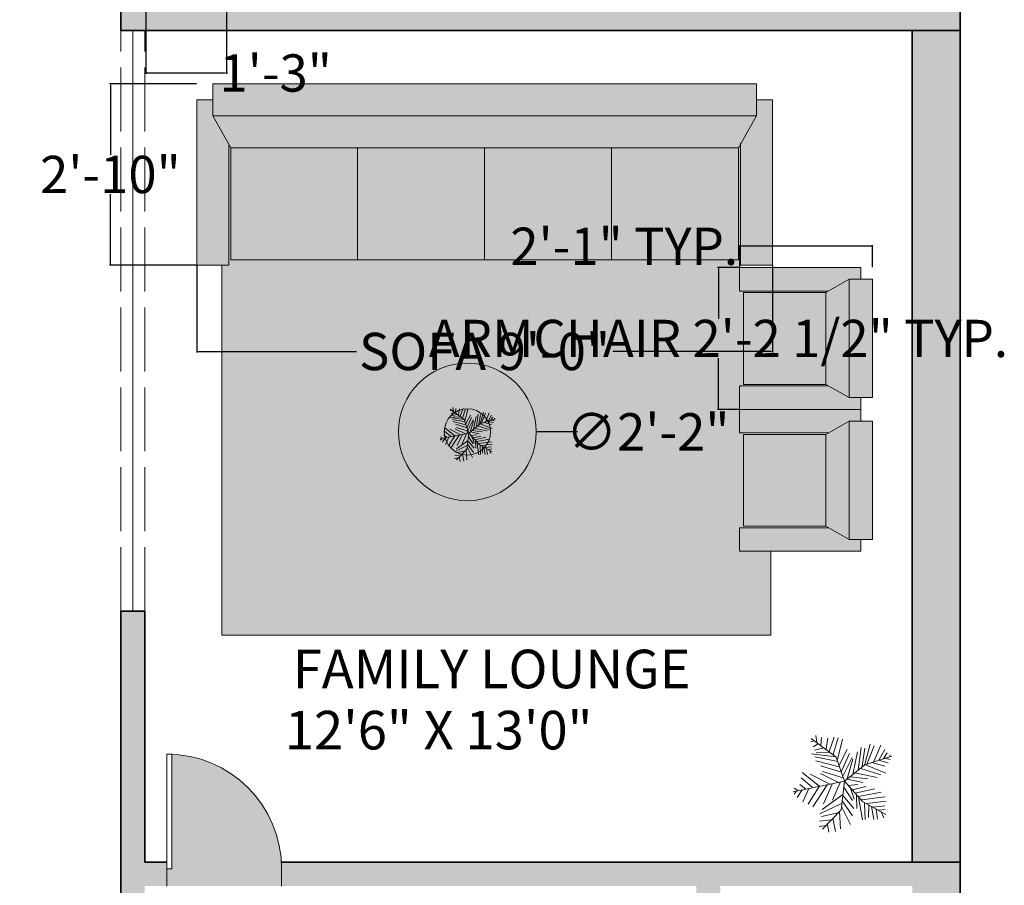
# Model space of a CAD drawing. Units: inches. Extents: x 2167 to 2589, y 1680 to 2489.
# Tile 33 of 38: x 2399 to 2583, y 1865 to 2027. Entities that reach past the tile are written whole.
import ezdxf

# ---------------------------------------------------------------- set-up
doc = ezdxf.new("R2010")
doc.units = ezdxf.units.IN
doc.header["$MEASUREMENT"] = 0
doc.linetypes.add('ACAD_ISO02W100', pattern=[15, 12, -3])
doc.layers.get('0').update_dxf_attribs({"color": 250})
for name, color, linetype, lineweight in [('A-ANNO-DIMS', 2, 'Continuous', 18), ('A-AREA-IDEN', 7, 'Continuous', 18), ('A-DOOR', 4, 'Continuous', 18), ('A-FURN-PATT', 31, 'Continuous', 13), ('A-WALL-OVHD', 8, 'ACAD_ISO02W100', 18), ('A-WALL-PATT', 250, 'Continuous', 13), ('C-PROP', 7, 'Continuous', 35), ('furniture', 34, 'Continuous', 18), ('L-PLNT', 106, 'Continuous', 13), ('walls', 7, 'Continuous', 35), ('windows', 141, 'Continuous', 18)]:
    doc.layers.add(name, color=color, linetype=linetype, lineweight=lineweight)
doc.layers.add('A-FLOR-PATT', color=254, linetype='Continuous', lineweight=13, true_color=0xfeeab9)
doc.styles.get("Standard").update_dxf_attribs({"font": 'arial.ttf'})
doc.dimstyles.get("Standard").update_dxf_attribs({"dimtxt": 7, "dimasz": 0.18, "dimexe": 0.18, "dimexo": 0.0625, "dimgap": 0.09, "dimtad": 0, "dimtih": 1, "dimtoh": 1, "dimdec": 1, "dimzin": 0, "dimdsep": 46, "dimlunit": 3, "dimtxsty": 'Standard', "dimcen": 0.09, "dimadec": 0, "dimazin": 0, "dimtfac": 1, "dimtdec": 1, "dimtofl": 0, "dimtmove": 0, "dimatfit": 3, "dimfxl": 1, "dimtolj": 1, "dimtzin": 0, "dimarcsym": 0})

# ---------------------------------------------------------------- blocks, each defined once
blk = doc.blocks.new('*U2')
for p, q in [((0, 0), (0, -6)), ((40, 0), (40, -6))]:
    blk.add_line(p, q)
blk.add_lwpolyline([(0, 0), (0, 40), (1.75, 40), (1.75, 0)], close=True)
blk.add_arc((0, 0), 40, 0, 90)
blk = doc.blocks.new('FABRIC SOFA 4S')
at = {"layer": 'furniture'}
for p, q in [((3, 54), (34, 54)), ((3, 51), (3, 54)), ((34, 48), (34, 54)), ((0, -51), (0, 51)), ((6, 51), (0, 51)), ((6, -51), (6, 51)), ((12, 47.63), (6, 51)), ((11.14, 48), (34, 48)), ((33, 23.81), (12, 23.81)), ((33, 0), (12, 0)), ((33, -23.81), (12, -23.81)), ((6, -51), (12, -47.63)), ((11.54, -48), (34, -48)), ((34, -48), (34, -54)), ((6, -51), (0, -51)), ((3, -54), (3, -51)), ((3, -54), (34, -54))]:
    blk.add_line(p, q, dxfattribs=at)
blk.add_lwpolyline([(12, -47.63), (12, 47.63), (33, 47.63), (33, -47.63)], close=True, dxfattribs=at)
blk = doc.blocks.new('FABRIC SOFA 1S')
at = {"layer": 'furniture'}
for p, q in [((3, 18.12), (34, 18.12)), ((3, 15.12), (3, 18.12)), ((34, 12.12), (34, 18.12)), ((0, -15.12), (0, 15.12)), ((6, 15.12), (0, 15.12)), ((6, -15.12), (6, 15.12)), ((12, 11.75), (6, 15.12)), ((11.33, 12.12), (34, 12.12)), ((6, -15.12), (12, -11.75)), ((11.33, -12.12), (34, -12.12)), ((34, -12.12), (34, -18.12)), ((6, -15.12), (0, -15.12)), ((3, -18.12), (3, -15.12)), ((3, -18.12), (34, -18.12))]:
    blk.add_line(p, q, dxfattribs=at)
blk.add_lwpolyline([(12, -11.75), (12, 11.75), (33, 11.75), (33, -11.75)], close=True, dxfattribs=at)
blk = doc.blocks.new('*U8')
for p, q in [((-10.186, 53.64), (-13.084, 55.962)), ((0, 0), (-10.5, 57)), ((-9.099, 51.782), (-6.563, 55.962)), ((-7.288, 39.707), (-21.778, 46.673)), ((-8.737, 47.138), (-17.069, 52.711)), ((-7.65, 43.423), (-2.578, 49.46)), ((-5.839, 35.992), (4.667, 48.067)), ((-5.114, 27.632), (10.463, 46.673)), ((-3.665, 19.273), (-27.574, 35.527)), ((-5.114, 28.097), (-24.676, 40.636)), ((-2.941, 16.486), (8.652, 37.85)), ((27, 9), (48, 36)), ((27.127, 9.056), (31.112, 35.992)), ((35.096, 32.741), (37.27, 22.524)), ((38.719, 34.134), (41.979, 28.561)), ((44.153, 36.456), (45.239, 32.741)), ((-31.5, 4.5), (-52.5, 25.5)), ((-48.585, 21.131), (-49.309, 29.026)), ((-43.513, 28.561), (-42.427, 15.558)), ((-38.442, 26.239), (-34.819, 7.663)), ((-35.544, 28.097), (-24.314, 3.947)), ((-14.533, 2.09), (-30.834, 25.31)), ((-24.314, 23.917), (-2.941, 13.7)), ((-1.129, 6.734), (9.014, 26.704)), ((3.942, 1.625), (11.187, 24.381)), ((10.101, 3.483), (17.708, 26.239)), ((16.259, 5.805), (23.142, 31.348)), ((22.055, 7.198), (27.489, 32.277)), ((31.836, 30.883), (32.561, 16.486)), ((40.53, 25.775), (48.862, 24.846)), ((43.791, 29.954), (51.036, 30.883)), ((-47.498, 19.737), (-55.83, 18.344)), ((-40.615, 13.7), (-55.105, 10.913)), ((-20.691, 13.7), (-1.129, 4.876)), ((29.662, 12.307), (48.137, 6.269)), ((33.285, 16.486), (48.862, 10.913)), ((36.183, 19.737), (48.137, 17.88)), ((-33.37, 6.269), (-52.207, 5.34)), ((-28.299, 3.483), (-47.86, -5.805)), ((-21.416, 3.018), (-38.079, -8.128)), ((0, 0), (-31.5, 4.5)), ((-15.982, 2.09), (-30.11, -9.521)), ((0, 0), (-22.5, -19.5)), ((-6.563, 1.161), (-21.416, -8.128)), ((0, 0), (27, 9)), ((0, 0), (18, -22.5)), ((6.478, 1.625), (26.04, -8.592)), ((11.187, 3.483), (30.749, -5.805)), ((18.07, 5.805), (35.096, -3.483)), ((24.229, 7.663), (46.688, 1.625)), ((-6.563, -5.805), (-19.967, -9.985)), ((-9.461, -8.592), (-6.201, -23.453)), ((-4.752, -3.483), (-3.665, -14.629)), ((2.493, -3.019), (-1.491, -20.202)), ((1.769, -2.555), (24.229, -9.521)), ((5.029, -6.27), (2.131, -25.775)), ((7.565, -9.056), (32.198, -14.629)), ((-17.431, -15.094), (-42.789, -18.809)), ((-24.314, -21.596), (-42.427, -22.06)), ((-22.5, -19.5), (-37.5, -45)), ((-15.257, -12.772), (-30.11, -12.772)), ((-20.691, -18.345), (-17.793, -44.352)), ((-17.069, -15.094), (-12.721, -40.172)), ((-13.446, -11.378), (-8.737, -32.741)), ((9.014, -11.378), (3.58, -35.992)), ((14.085, -16.951), (6.478, -40.172)), ((12.274, -15.094), (36.907, -18.809)), ((16.259, -19.738), (36.183, -22.989)), ((-28.299, -29.026), (-42.789, -31.348)), ((-26.849, -26.24), (-40.253, -25.775)), ((-29.023, -30.884), (-27.936, -43.887)), ((-25.038, -23.918), (-22.865, -45.281)), ((18.07, -22.524), (8.289, -45.745)), ((20.244, -30.419), (15.897, -44.816)), ((18, -22.5), (27, -52.5)), ((18.433, -22.524), (40.53, -29.026)), ((19.157, -25.311), (38.719, -33.206)), ((-30.834, -34.135), (-42.427, -35.528)), ((-34.457, -39.708), (-40.978, -42.494)), ((-32.646, -36.921), (-31.921, -44.352)), ((22.78, -37.85), (19.519, -48.532)), ((21.331, -32.741), (39.081, -40.636)), ((22.78, -38.314), (34.372, -44.816)), ((24.591, -43.423), (30.749, -47.603)), ((24.591, -45.745), (23.142, -50.854)), ((26.764, -49.925), (28.213, -50.854))]:
    blk.add_line(p, q)
blk = doc.blocks.new('*D27')
at = {"layer": 'A-ANNO-DIMS', "color": 0, "lineweight": -2, "transparency": 16777216}
for p, q in [((2533.62, 1980.71), (2529.51, 1980.71)), ((2529.69, 1980.53), (2529.69, 1971.12)), ((2529.69, 1954.28), (2529.69, 1963.7)), ((2533.62, 1954.1), (2529.51, 1954.1))]:
    blk.add_line(p, q, dxfattribs=at)
at = {"layer": 'A-ANNO-DIMS', "color": 0, "transparency": 16777216}
for points in [[(2529.66, 1980.53), (2529.72, 1980.53), (2529.69, 1980.71)], [(2529.66, 1954.28), (2529.72, 1954.28), (2529.69, 1954.1)]]:
    blk.add_solid(points, dxfattribs=at)
at = {"layer": 'Defpoints', "color": 0, "transparency": 16777216}
for p in [(2533.68, 1980.71), (2529.69, 1954.1), (2533.68, 1954.1)]:
    blk.add_point(p, dxfattribs=at)
at = {"layer": 'A-ANNO-DIMS', "color": 0, "transparency": 16777216, "insert": (2529.69, 1967.41), "char_height": 7, "attachment_point": 5}
blk.add_mtext('\\A1;ARMCHAIR 2\'-2 1/2" TYP.', dxfattribs=at)
blk = doc.blocks.new('*D28')
at = {"layer": 'A-ANNO-DIMS', "color": 0, "lineweight": -2, "transparency": 16777216}
for p, q in [((2533.68, 1984.7), (2533.5, 1984.7)), ((2533.68, 1980.77), (2533.68, 1984.88)), ((2558.45, 1984.7), (2533.86, 1984.7)), ((2558.63, 1980.77), (2558.63, 1984.88))]:
    blk.add_line(p, q, dxfattribs=at)
at = {"layer": 'A-ANNO-DIMS', "color": 0, "transparency": 16777216}
for points in [[(2533.86, 1984.73), (2533.86, 1984.67), (2533.68, 1984.7)], [(2558.45, 1984.73), (2558.45, 1984.67), (2558.63, 1984.7)]]:
    blk.add_solid(points, dxfattribs=at)
at = {"layer": 'Defpoints', "color": 0, "transparency": 16777216}
for p in [(2533.68, 1984.7), (2533.68, 1980.71), (2558.63, 1980.71)]:
    blk.add_point(p, dxfattribs=at)
at = {"layer": 'A-ANNO-DIMS', "color": 0, "transparency": 16777216, "insert": (2512.01, 1984.7), "char_height": 7, "attachment_point": 5}
blk.add_mtext('\\A1;2\'-1" TYP.', dxfattribs=at)
blk = doc.blocks.new('*D36')
at = {"layer": 'A-ANNO-DIMS', "color": 0, "lineweight": -2, "transparency": 16777216}
for p, q in [((2422.24, 2029.15), (2422.24, 2017.03)), ((2437.38, 2029.15), (2437.38, 2017.03)), ((2422.42, 2017.21), (2437.2, 2017.21)), ((2437.38, 2017.21), (2437.56, 2017.21))]:
    blk.add_line(p, q, dxfattribs=at)
at = {"layer": 'A-ANNO-DIMS', "color": 0, "transparency": 16777216}
for points in [[(2422.42, 2017.24), (2422.42, 2017.18), (2422.24, 2017.21)], [(2437.2, 2017.24), (2437.2, 2017.18), (2437.38, 2017.21)]]:
    blk.add_solid(points, dxfattribs=at)
at = {"layer": 'Defpoints', "color": 0, "transparency": 16777216}
for p in [(2422.24, 2029.21), (2437.38, 2029.21), (2437.38, 2017.21)]:
    blk.add_point(p, dxfattribs=at)
at = {"layer": 'A-ANNO-DIMS', "color": 0, "transparency": 16777216, "insert": (2446.62, 2017.21), "char_height": 7, "attachment_point": 5}
blk.add_mtext('\\A1;1\'-3"', dxfattribs=at)
blk = doc.blocks.new('*D41')
at = {"layer": 'A-ANNO-DIMS', "color": 0, "lineweight": -2, "transparency": 16777216}
for p, q in [((2431.81, 1981.11), (2431.81, 1964.79)), ((2539.81, 1981.11), (2539.81, 1964.79)), ((2431.99, 1964.97), (2461.76, 1964.97)), ((2539.63, 1964.97), (2509.86, 1964.97))]:
    blk.add_line(p, q, dxfattribs=at)
at = {"layer": 'A-ANNO-DIMS', "color": 0, "transparency": 16777216}
for points in [[(2431.99, 1965), (2431.99, 1964.94), (2431.81, 1964.97)], [(2539.63, 1965), (2539.63, 1964.94), (2539.81, 1964.97)]]:
    blk.add_solid(points, dxfattribs=at)
at = {"layer": 'Defpoints', "color": 0, "transparency": 16777216}
for p in [(2431.81, 1981.17), (2539.81, 1981.17), (2539.81, 1964.97)]:
    blk.add_point(p, dxfattribs=at)
at = {"layer": 'A-ANNO-DIMS', "color": 0, "transparency": 16777216, "insert": (2485.81, 1964.97), "char_height": 7, "attachment_point": 5}
blk.add_mtext('\\A1;SOFA 9\'-0"', dxfattribs=at)
blk = doc.blocks.new('*D42')
at = {"layer": 'A-ANNO-DIMS', "color": 0, "lineweight": -2, "transparency": 16777216}
for p, q in [((2431.75, 2015.17), (2415.43, 2015.17)), ((2415.61, 2014.99), (2415.61, 2001.83)), ((2415.61, 1981.35), (2415.61, 1994.5)), ((2431.75, 1981.17), (2415.43, 1981.17))]:
    blk.add_line(p, q, dxfattribs=at)
at = {"layer": 'A-ANNO-DIMS', "color": 0, "transparency": 16777216}
for points in [[(2415.58, 2014.99), (2415.64, 2014.99), (2415.61, 2015.17)], [(2415.58, 1981.35), (2415.64, 1981.35), (2415.61, 1981.17)]]:
    blk.add_solid(points, dxfattribs=at)
at = {"layer": 'Defpoints', "color": 0, "transparency": 16777216}
for p in [(2431.81, 2015.17), (2415.61, 1981.17), (2431.81, 1981.17)]:
    blk.add_point(p, dxfattribs=at)
at = {"layer": 'A-ANNO-DIMS', "color": 0, "transparency": 16777216, "insert": (2415.61, 1998.17), "char_height": 7, "attachment_point": 5}
blk.add_mtext('\\A1;2\'-10"', dxfattribs=at)
blk = doc.blocks.new('*D59')
at = {"layer": 'A-ANNO-DIMS', "color": 0, "lineweight": -2, "transparency": 16777216}
for p, q in [((2482.5, 1949.89), (2482.68, 1949.89)), ((2482.59, 1949.8), (2482.59, 1949.98)), ((2503.25, 1949.89), (2495.68, 1949.89))]:
    blk.add_line(p, q, dxfattribs=at)
at = {"layer": 'A-ANNO-DIMS', "color": 0, "transparency": 16777216}
blk.add_solid([(2495.68, 1949.92), (2495.68, 1949.86), (2495.5, 1949.89)], dxfattribs=at)
at = {"layer": 'Defpoints', "color": 0, "transparency": 16777216}
for p in [(2469.68, 1949.89), (2495.5, 1949.89)]:
    blk.add_point(p, dxfattribs=at)
at = {"layer": 'A-ANNO-DIMS', "color": 0, "transparency": 16777216, "insert": (2516.45, 1949.89), "char_height": 7, "attachment_point": 5}
blk.add_mtext('\\A1;∅2\'-2"', dxfattribs=at)

msp = doc.modelspace()

# ---------------------------------------------------------------- hatches: boundary and pattern name
at = {"layer": 'A-FLOR-PATT'}
h = msp.add_hatch(color=256, dxfattribs=at)
h.dxf.hatch_style = 1
h.paths.add_polyline_path([(2427.15, 1889.43), (2427.15, 1867.92), (2426.21, 1867.92), (2426.21, 1864.69), (2447.74, 1864.69), (2447.74, 1867.92, 0.401453)])
at = {"layer": 'A-FURN-PATT'}
h = msp.add_hatch(color=256, dxfattribs=at)
h.dxf.hatch_style = 1
h.paths.add_polyline_path([(2533.43, 1982.17), (2533.43, 2003.17), (2509.62, 2003.17), (2509.62, 1982.17)])
h.paths.add_polyline_path([(2509.62, 1982.17), (2509.62, 2003.17), (2485.81, 2003.17), (2485.81, 1982.17)])
h.paths.add_polyline_path([(2485.81, 1982.17), (2485.81, 2003.17), (2462, 2003.17), (2462, 1982.17)])
h.paths.add_polyline_path([(2462, 1982.17), (2462, 2003.17), (2438.18, 2003.17), (2438.18, 1982.17)])
h.paths.add_polyline_path([(2533.43, 2003.17), (2536.81, 2009.17), (2434.81, 2009.17), (2438.18, 2003.17)])
h.paths.add_polyline_path([(2536.81, 2009.17), (2536.81, 2015.17), (2434.81, 2015.17), (2434.81, 2009.17)])
h.paths.add_polyline_path([(2539.81, 1981.17), (2539.81, 2012.17), (2536.81, 2012.17), (2536.81, 2009.17), (2533.81, 2003.84), (2533.81, 1981.17)])
h.paths.add_polyline_path([(2437.81, 1981.17), (2437.81, 2003.84), (2434.81, 2009.17), (2434.81, 2012.17), (2431.81, 2012.17), (2431.81, 1981.17)])
h = msp.add_hatch(color=256, dxfattribs=at)
h.dxf.hatch_style = 1
h.paths.add_polyline_path([(2539.5, 1927.5), (2533.68, 1927.5), (2533.68, 1931.9), (2534.41, 1931.9), (2534.41, 1949.7), (2533.68, 1949.7), (2533.68, 1954.1), (2533.68, 1958.51), (2534.41, 1958.51), (2534.41, 1976.31), (2533.68, 1976.31), (2533.68, 1981.17), (2533.81, 1981.17), (2533.81, 2003.84), (2536.81, 2009.17), (2434.81, 2009.17), (2437.81, 2003.84), (2437.81, 1981.17), (2436.54, 1981.17), (2436.54, 1911.78), (2539.5, 1911.78)])
h.paths.add_polyline_path([(2469.68, 1949.89, -1), (2495.5, 1949.89, -1)], flags=16)
h.paths.add_polyline_path([(2478.25, 1949.89, -1), (2486.92, 1949.89, -1)], flags=0)
h.paths.add_polyline_path([(2533.43, 1982.17), (2438.18, 1982.17), (2438.18, 2003.17), (2533.43, 2003.17)], flags=16)
h = msp.add_hatch(color=256, dxfattribs=at)
h.dxf.hatch_style = 1
h.paths.add_polyline_path([(2549.83, 1976.03), (2534.41, 1976.03), (2534.41, 1958.78), (2549.83, 1958.78)])
h.paths.add_polyline_path([(2554.23, 1978.51), (2556.43, 1978.51), (2556.43, 1980.71), (2533.68, 1980.71), (2533.68, 1976.31), (2550.31, 1976.31)])
h.paths.add_polyline_path([(2558.63, 1978.51), (2554.23, 1978.51), (2554.23, 1956.31), (2558.63, 1956.31)])
h.paths.add_polyline_path([(2554.23, 1978.51), (2549.83, 1976.03), (2549.83, 1958.78), (2554.23, 1956.31)])
h.paths.add_polyline_path([(2550.31, 1958.51), (2533.68, 1958.51), (2533.68, 1954.1), (2556.43, 1954.1), (2556.43, 1956.31), (2554.23, 1956.31)])
h.paths.add_polyline_path([(2554.23, 1951.9), (2556.43, 1951.9), (2556.43, 1954.1), (2533.68, 1954.1), (2533.68, 1949.7), (2550.31, 1949.7)])
h.paths.add_polyline_path([(2554.23, 1951.9), (2549.83, 1949.42), (2549.83, 1932.18), (2554.23, 1929.7)])
h.paths.add_polyline_path([(2558.63, 1951.9), (2554.23, 1951.9), (2554.23, 1929.7), (2558.63, 1929.7)])
h.paths.add_polyline_path([(2549.83, 1949.42), (2534.41, 1949.42), (2534.41, 1932.18), (2549.83, 1932.18)])
h.paths.add_polyline_path([(2550.31, 1931.9), (2533.68, 1931.9), (2533.68, 1927.5), (2556.43, 1927.5), (2556.43, 1929.7), (2554.23, 1929.7)])
h = msp.add_hatch(color=256, dxfattribs=at)
h.dxf.hatch_style = 1
h.paths.add_polyline_path([(2469.68, 1949.89, 1), (2495.5, 1949.89, 1)])
h.paths.add_polyline_path([(2486.92, 1949.89, -1), (2478.25, 1949.89, -1)], flags=16)
h = msp.add_hatch(color=256, dxfattribs=at)
h.dxf.hatch_style = 1
h.paths.add_polyline_path([(2481.99, 1952.22), (2480.24, 1953.53, 0.254992), (2478.25, 1949.89, 0.066123), (2478.4, 1948.76), (2482.89, 1949.66)])
h.paths.add_polyline_path([(2480.24, 1953.53), (2481.67, 1952.46), (2482.2, 1954.21, 0.121407)])
h.paths.add_polyline_path([(2482.2, 1954.21), (2481.67, 1952.46), (2481.99, 1952.22), (2482.89, 1949.66), (2485.01, 1951.42), (2485.02, 1951.42), (2486.44, 1951.87, 0.304952)])
h.paths.add_polyline_path([(2482.89, 1949.66), (2484.79, 1947.55), (2485.2, 1947.32), (2486.16, 1947.43, 0.151975), (2486.92, 1949.89, 0.046128), (2486.85, 1950.68), (2485.02, 1951.42), (2485.01, 1951.42)])
h.paths.add_polyline_path([(2486.44, 1951.87), (2485.02, 1951.42), (2486.85, 1950.68, 0.072952)])
h.paths.add_polyline_path([(2482.89, 1949.66), (2480.22, 1949.12), (2479.1, 1947.31, 0.119517), (2480.67, 1946), (2482.2, 1946.33), (2482.51, 1946.65)])
h.paths.add_polyline_path([(2480.22, 1949.12), (2479.12, 1948.9), (2478.7, 1947.98, 0.045206), (2479.1, 1947.31)])
h.paths.add_polyline_path([(2479.12, 1948.9), (2478.42, 1948.76), (2478.41, 1948.75, 0.047094), (2478.7, 1947.98)])
h.paths.add_polyline_path([(2482.2, 1946.33), (2480.67, 1946, 0.055414), (2481.57, 1945.68)])
h.paths.add_polyline_path([(2482.35, 1946.48), (2481.65, 1945.76), (2481.68, 1945.65, 0.04264), (2482.41, 1945.56)])
h.paths.add_polyline_path([(2484.68, 1946.09), (2484.36, 1948.03), (2482.89, 1949.66), (2482.51, 1946.65), (2482.35, 1946.48), (2482.41, 1945.56, 0.136795)])
h.paths.add_polyline_path([(2485.8, 1946.98), (2484.79, 1947.55), (2484.36, 1948.03), (2484.68, 1946.09, 0.08323)])
h.paths.add_polyline_path([(2486.16, 1947.43), (2485.2, 1947.32), (2485.8, 1946.98, 0.033271)])
at = {"layer": 'A-WALL-PATT'}
h = msp.add_hatch(color=256, dxfattribs=at)
h.dxf.hatch_style = 1
h.paths.add_polyline_path([(2575.05, 2029.69), (2422.05, 2029.69), (2422.05, 2161.69), (2427.02, 2161.69), (2427.02, 2161.94), (2427.02, 2166.19), (2417.55, 2166.19), (2417.55, 2025.19), (2575.05, 2025.19)])
h.paths.add_polyline_path([(2575.05, 2166.19), (2503.01, 2166.19), (2503.01, 2161.69), (2575.05, 2161.69)], flags=17)
h.paths.add_polyline_path([(2575.05, 2161.69), (2566.05, 2161.69), (2566.05, 2029.69), (2575.05, 2029.69)], flags=17)
h.paths.add_polyline_path([(2575.05, 2025.19), (2566.05, 2025.19), (2566.05, 1869.19), (2575.05, 1869.19)])
h.paths.add_polyline_path([(2575.05, 1869.19), (2566.05, 1869.19), (2447.7, 1869.19, -0.014764), (2447.74, 1867.92), (2447.74, 1864.69), (2575.05, 1864.69)])
h.paths.add_polyline_path([(2530.05, 1864.69), (2525.55, 1864.69), (2525.55, 1816.69), (2452.05, 1816.69), (2452.05, 1812.19), (2530.05, 1812.19)])
h.paths.add_polyline_path([(2455.04, 1830.65), (2452.05, 1830.65), (2452.05, 1816.69), (2455.04, 1816.69)], flags=17)
h.paths.add_polyline_path([(2575.05, 1864.69), (2566.05, 1864.69), (2566.05, 1788.19), (2456.1, 1788.19), (2456.1, 1783.94, -0.042065), (2455.7, 1779.19), (2527.68, 1779.19), (2527.68, 1687.69), (2532.18, 1687.69), (2532.18, 1779.19), (2575.05, 1779.19)])
h.paths.add_polyline_path([(2421.87, 1696.69), (2416.11, 1696.69), (2416.11, 1687.69), (2421.87, 1687.69)])
h.paths.add_polyline_path([(2375.61, 1696.69), (2369.84, 1696.69), (2369.84, 1687.69), (2375.61, 1687.69)])
h.paths.add_polyline_path([(2425.05, 2245.69), (2420.55, 2245.69), (2420.55, 2226.19), (2432.29, 2226.19), (2432.29, 2229.42), (2432.29, 2230.69), (2425.05, 2230.69)])
h.paths.add_polyline_path([(2224.05, 2151.19), (2318.55, 2151.19), (2318.55, 2177.3), (2314.78, 2177.3, -0.007324), (2314.05, 2177.32), (2314.05, 2155.69), (2224.05, 2155.69), (2224.05, 2157.46), (2215.05, 2157.46), (2215.05, 2103.59), (2218.97, 2103.59), (2224.05, 2103.59)])
h = msp.add_hatch(color=256, dxfattribs=at)
h.dxf.hatch_style = 1
h.paths.add_polyline_path([(2274.74, 1855.04), (2224.05, 1855.04), (2224.05, 2003.12), (2215.05, 2003.12), (2215.05, 1846.04), (2274.74, 1846.04)])
h.paths.add_polyline_path([(2354.89, 1855.04), (2330.89, 1855.04), (2330.89, 1846.04), (2354.77, 1846.04), (2354.77, 1852.04, -0.01877)])
h.paths.add_polyline_path([(2422.05, 1864.69), (2426.21, 1864.69), (2426.21, 1867.92), (2426.21, 1869.19), (2422.05, 1869.19), (2422.05, 1916.24), (2417.55, 1916.24), (2417.55, 1855.04), (2394.77, 1855.04), (2394.77, 1852.04), (2394.77, 1846.04), (2417.55, 1846.04), (2417.55, 1779.19), (2427.74, 1779.19), (2427.74, 1783.94), (2427.74, 1788.19), (2422.05, 1788.19)])

# ---------------------------------------------------------------- linework, layer by layer
at = {"layer": 'A-WALL-OVHD'}
for p, q in [((2417.55, 1916.24), (2417.55, 2025.19)), ((2422.05, 1916.24), (2422.05, 2025.19))]:
    msp.add_line(p, q, dxfattribs=at)
at = {"layer": 'C-PROP'}
msp.add_line((2575.05, 2407.69), (2575.05, 1687.69), dxfattribs=at)
at = {"layer": 'furniture'}
for p, q in [((2436.54, 1911.78), (2436.54, 1981.17)), ((2539.5, 1927.5), (2539.5, 1911.78)), ((2539.5, 1911.78), (2436.54, 1911.78))]:
    msp.add_line(p, q, dxfattribs=at)
for radius in [12.91, 4.34]:
    msp.add_circle((2482.59, 1949.89), radius, dxfattribs=at)
at = {"layer": 'walls'}
for p, q in [((2417.55, 2166.19), (2417.55, 2025.19)), ((2417.55, 2025.19), (2575.05, 2025.19)), ((2566.05, 2025.19), (2566.05, 1869.19)), ((2417.55, 1916.24), (2422.05, 1916.24)), ((2417.55, 1916.24), (2417.55, 1855.04)), ((2422.05, 1916.24), (2422.05, 1869.19)), ((2422.05, 1869.19), (2426.21, 1869.19)), ((2447.7, 1869.19), (2575.05, 1869.19))]:
    msp.add_line(p, q, dxfattribs=at)
at = {"layer": 'windows'}
msp.add_line((2419.8, 1916.24), (2419.8, 2025.19), dxfattribs=at)

# ---------------------------------------------------------------- block references
at = {"layer": 'A-DOOR', "xscale": 0.5382298898187942, "yscale": 0.5382298898187942, "zscale": 0.5382298898187942}
msp.add_blockref('*U2', (2426.21, 1867.92), dxfattribs=at)
at = {"layer": 'furniture', "rotation": 270}
msp.add_blockref('FABRIC SOFA 4S', (2485.81, 2015.17), dxfattribs=at)
at = {"layer": 'furniture', "xscale": 0.7339463821036302, "yscale": 0.7339463821036302, "zscale": 0.7339463821036302}
for p, rotation in [((2558.63, 1967.41), 180), ((2558.63, 1940.8), 180.0000000000007)]:
    msp.add_blockref('FABRIC SOFA 1S', p, dxfattribs=dict(at, rotation=rotation))
at = {"layer": 'L-PLNT', "rotation": 90.98387132377816}
for p, xscale, yscale, zscale in [((2482.89, 1949.66), 0.0953220490742722, 0.0953220490742722, 0.0953220490742722), ((2553.38, 1884.34), 0.1698531738429223, 0.1698531738429223, 0.1698531738429223)]:
    msp.add_blockref('*U8', p, dxfattribs=dict(at, xscale=xscale, yscale=yscale, zscale=zscale))

# ---------------------------------------------------------------- texts
at = {"layer": 'A-AREA-IDEN'}
for s, p in [('FAMILY LOUNGE', (2449.82, 1901.8)), ('12\'6" X 13\'0"', (2448.34, 1890.33))]:
    msp.add_text(s, height=7.2272, dxfattribs=at).set_placement(p)

# ---------------------------------------------------------------- dimensions: what is measured, and where the dimension line sits
at = {"layer": 'A-ANNO-DIMS'}
dim = msp.add_linear_dim(base=(2437.38, 2017.21), p1=(2422.24, 2029.21), p2=(2437.38, 2029.21), dimstyle='Standard', override={"dimdec": 1, "dimlfac": 1, "dimrnd": 0, "dimzin": 1, "dimdsep": 46, "dimlunit": 4, "dimfrac": 2}, dxfattribs=at)
dim.commit()
dim.dimension.update_dxf_attribs({"geometry": '*D36', "text_midpoint": (2446.62, 2017.21)})
dim = msp.add_linear_dim(base=(2415.61, 1981.17), p1=(2431.81, 2015.17), p2=(2431.81, 1981.17), angle=270, dimstyle='Standard', override={"dimdec": 1, "dimlfac": 1, "dimrnd": 0, "dimzin": 1, "dimdsep": 46, "dimlunit": 4, "dimfrac": 2}, dxfattribs=at)
dim.commit()
dim.dimension.update_dxf_attribs({"geometry": '*D42', "text_midpoint": (2415.61, 1998.17)})
for base, p1, p2, angle, text, picture, middle in [((2533.6787, 1984.6997), (2558.6329, 1980.7088), (2533.6787, 1980.7088), 180, '<> TYP.', '*D28', (2512.0148, 1984.6997)), ((2529.69, 1954.1), (2533.68, 1980.71), (2533.68, 1954.1), 270, 'ARMCHAIR <> TYP.', '*D27', (2529.69, 1967.41))]:
    dim = msp.add_linear_dim(base=base, p1=p1, p2=p2, angle=angle, text=text, dimstyle='Standard', override={"dimdec": 1, "dimlfac": 1, "dimrnd": 0, "dimzin": 1, "dimdsep": 46, "dimlunit": 4, "dimfrac": 2}, dxfattribs=at)
    dim.commit()
    dim.dimension.update_dxf_attribs({"geometry": picture, "text_midpoint": middle})
dim = msp.add_linear_dim(base=(2539.81, 1964.97), p1=(2431.81, 1981.17), p2=(2539.81, 1981.17), text='SOFA <>', dimstyle='Standard', override={"dimdec": 1, "dimlfac": 1, "dimrnd": 0, "dimzin": 1, "dimdsep": 46, "dimlunit": 4, "dimfrac": 2}, dxfattribs=at)
dim.commit()
dim.dimension.update_dxf_attribs({"geometry": '*D41', "text_midpoint": (2485.81, 1964.97)})
dim = msp.add_diameter_dim_2p(p1=(2469.68, 1949.89), p2=(2495.5, 1949.89), dimstyle='Standard', override={"dimdec": 1, "dimlfac": 1, "dimrnd": 0, "dimzin": 1, "dimdsep": 46, "dimlunit": 4, "dimfrac": 2}, dxfattribs=at)
dim.commit()
dim.dimension.update_dxf_attribs({"geometry": '*D59', "text_midpoint": (2503.25, 1949.89), "dimtype": 163})

doc.saveas('drawing.dxf')
